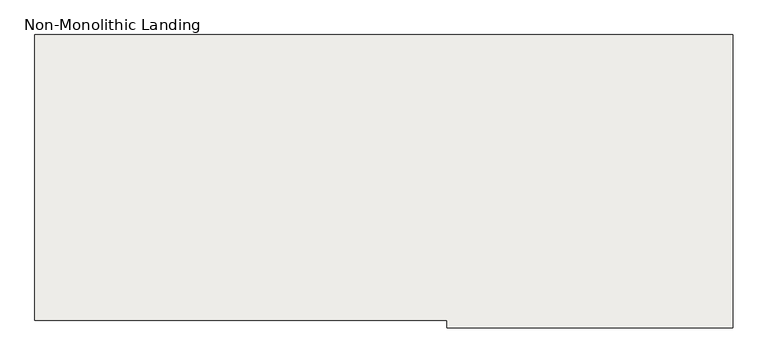
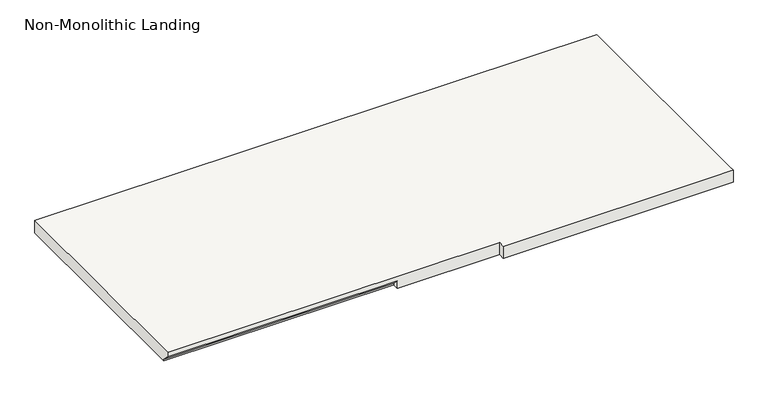
"""IFC4 building model written with IfcOpenShell, lengths in millimetres: slab geometry, Non-Monolithic Landing."""

from ifc_helpers import new_model, si_unit, origin, place, context, project, spatial, faceted_brep, source, transform, mapped, element, save


def non_monolithic_landing_1beb21ea(model_context):
    return source(origin(), model_context, "Body", "Brep", [
        faceted_brep([(-3617.4415084, -19522.1851539, 39778.2339133), (-3617.4415084, -19496.7851539, 39752.8339133), (-2703.0415084, -19496.7851539, 39752.8339133), (-2703.0415084, -19522.1851539, 39778.2339133), (-2296.6415084, -19522.1851539, 39797.2839133), (-2296.6415084, -19547.5851539, 39797.2839133), (-1382.2415084, -19547.5851539, 39797.2839133), (-1382.2415084, -19522.1851539, 39797.2839133), (-1382.2415084, -18607.7851539, 39797.2839133), (-3617.4415084, -18607.7851539, 39797.2839133), (-3617.4415084, -19522.1851539, 39797.2839133), (-2703.0415084, -19496.7851539, 39746.4839133), (-3617.4415084, -19496.7851539, 39746.4839133), (-3617.4415084, -18607.7851539, 39746.4839133), (-1382.2415084, -18607.7851539, 39746.4839133), (-1382.2415084, -19522.1851539, 39746.4839133), (-1382.2415084, -19547.5851539, 39746.4839133), (-2296.6415084, -19547.5851539, 39746.4839133), (-2296.6415084, -19522.1851539, 39746.4839133), (-2703.0415084, -19522.1851539, 39746.4839133)], [[[0, 1, 2, 3]], [[4, 5, 6, 7, 8, 9, 10]], [[11, 12, 13, 14, 15, 16, 17, 18, 19]], [[12, 11, 2, 1]], [[11, 19, 3, 2]], [[4, 10, 0, 3, 19, 18]], [[5, 4, 18, 17]], [[6, 5, 17, 16]], [[7, 6, 16, 15]], [[8, 7, 15, 14]], [[9, 8, 14, 13]], [[10, 9, 13, 12, 1, 0]]]),
    ])


if __name__ == "__main__":
    model = new_model("IFC4")
    model_context = context("Model", 3, world=origin())
    ifc_project = project(units=[si_unit("LENGTHUNIT", "METRE", prefix="MILLI")], contexts=[model_context])
    site = spatial("IfcSite", under=ifc_project)
    building = spatial("IfcBuilding", under=site)
    placement = place(None, origin())
    non_monolithic_landing_shape = non_monolithic_landing_1beb21ea(model_context)
    element("IfcSlab", 1, ObjectType="Non-Monolithic Landing", at=placement, inside=building, context=model_context, shape_type="MappedRepresentation", body=[
        mapped(non_monolithic_landing_shape, transform((0.0, 0.0, 0.0), x_axis=(1.0, 0.0, 0.0), y_axis=(0.0, 1.0, 0.0), z_axis=(0.0, 0.0, 1.0))),
    ])
    save(model, "model.ifc")
